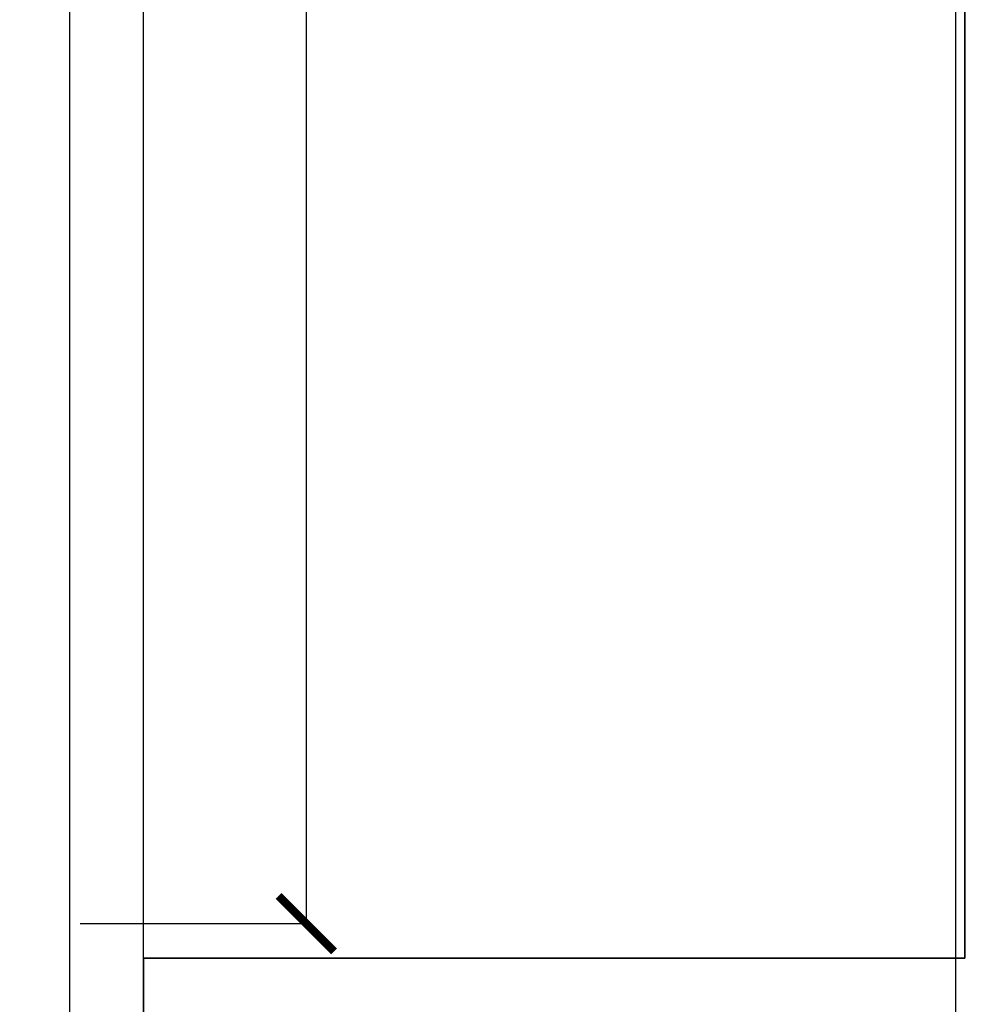
# Model space of a CAD drawing. Units: inches. Extents: x 844 to 2234, y 346 to 1084.
# Tile 6 of 93: x 1136 to 1189, y 627 to 680. Entities that reach past the tile are written whole.
import ezdxf

# ---------------------------------------------------------------- set-up
doc = ezdxf.new("R2010")
doc.units = ezdxf.units.IN
doc.header["$MEASUREMENT"] = 0
doc.layers.add('A-ANNO-DIMS', color=2, linetype='Continuous', lineweight=18)
doc.layers.add('A-WALL', color=7, linetype='Continuous', lineweight=35)
doc.styles.get("Standard").update_dxf_attribs({"font": 'arial.ttf'})
doc.dimstyles.get("Standard").update_dxf_attribs({"dimtxt": 6, "dimasz": 3, "dimexe": 0.18, "dimexo": 0.0625, "dimgap": 0.09, "dimtad": 0, "dimtih": 1, "dimtoh": 1, "dimdec": 1, "dimzin": 0, "dimdsep": 46, "dimlunit": 3, "dimtxsty": 'Standard', "dimblk": 'ARCHTICK', "dimcen": 0.09, "dimadec": 0, "dimazin": 0, "dimtfac": 1, "dimtdec": 1, "dimtofl": 0, "dimtmove": 0, "dimatfit": 3, "dimfxl": 1, "dimtolj": 1, "dimtzin": 0, "dimarcsym": 0})

# ---------------------------------------------------------------- blocks, each defined once
blk = doc.blocks.new('_ArchTick')
at = {"color": 0, "linetype": 'ByBlock', "const_width": 0.15}
blk.add_lwpolyline([(-0.5, -0.5), (0.5, 0.5)], dxfattribs=at)
blk = doc.blocks.new('*D54')
at = {"layer": 'A-ANNO-DIMS', "color": 0, "lineweight": -2, "transparency": 16777216}
for p, q in [((1139.678, 879.311), (1152.117, 879.311)), ((1151.937, 879.311), (1151.937, 758.401)), ((1151.937, 631.184), (1151.937, 752.094)), ((1139.678, 631.184), (1152.117, 631.184))]:
    blk.add_line(p, q, dxfattribs=at)
at = {"layer": 'Defpoints', "color": 0, "transparency": 16777216}
for p in [(1139.616, 879.311), (1139.616, 631.184), (1151.937, 631.184)]:
    blk.add_point(p, dxfattribs=at)
at = {"layer": 'A-ANNO-DIMS', "color": 0, "lineweight": -2, "transparency": 16777216, "xscale": 3, "yscale": 3, "zscale": 3}
for p, rotation in [((1151.937, 879.311), 90), ((1151.937, 631.184), 270)]:
    blk.add_blockref('_ArchTick', p, dxfattribs=dict(at, rotation=rotation))
at = {"layer": 'A-ANNO-DIMS', "color": 0, "transparency": 16777216, "insert": (1151.937, 755.248), "char_height": 6, "attachment_point": 5}
blk.add_mtext('\\A1;20\'-8.1"', dxfattribs=at)
blk = doc.blocks.new('*D143')
at = {"layer": 'A-ANNO-DIMS', "color": 0, "lineweight": -2, "transparency": 16777216}
for p, q in [((1139.116, 430.373), (1139.116, 1074.743)), ((1187.116, 430.373), (1187.116, 1074.743)), ((1139.116, 1074.563), (1154.93, 1074.563)), ((1187.116, 1074.563), (1171.301, 1074.563))]:
    blk.add_line(p, q, dxfattribs=at)
at = {"layer": 'Defpoints', "color": 0, "transparency": 16777216}
for p in [(1187.116, 1074.563), (1139.116, 430.311), (1187.116, 430.311)]:
    blk.add_point(p, dxfattribs=at)
at = {"layer": 'A-ANNO-DIMS', "color": 0, "lineweight": -2, "transparency": 16777216, "xscale": 3, "yscale": 3, "zscale": 3, "rotation": 180}
blk.add_blockref('_ArchTick', (1139.116, 1074.563), dxfattribs=at)
at = {"layer": 'A-ANNO-DIMS', "color": 0, "lineweight": -2, "transparency": 16777216, "xscale": 3, "yscale": 3, "zscale": 3}
blk.add_blockref('_ArchTick', (1187.116, 1074.563), dxfattribs=at)
at = {"layer": 'A-ANNO-DIMS', "color": 0, "transparency": 16777216, "insert": (1163.116, 1074.563), "char_height": 6, "attachment_point": 5}
blk.add_mtext('\\A1;4\'-0"', dxfattribs=at)
blk = doc.blocks.new('*D144')
at = {"layer": 'A-ANNO-DIMS', "color": 0, "lineweight": -2, "transparency": 16777216}
for p, q in [((1096.616, 439.373), (1096.616, 1074.743)), ((1143.116, 492.373), (1143.116, 1074.743)), ((1096.616, 1074.563), (1102.482, 1074.563)), ((1143.116, 1074.563), (1137.25, 1074.563))]:
    blk.add_line(p, q, dxfattribs=at)
at = {"layer": 'Defpoints', "color": 0, "transparency": 16777216}
for p in [(1143.116, 1074.563), (1143.116, 492.311), (1096.616, 439.311)]:
    blk.add_point(p, dxfattribs=at)
at = {"layer": 'A-ANNO-DIMS', "color": 0, "lineweight": -2, "transparency": 16777216, "xscale": 3, "yscale": 3, "zscale": 3, "rotation": 180}
blk.add_blockref('_ArchTick', (1096.616, 1074.563), dxfattribs=at)
at = {"layer": 'A-ANNO-DIMS', "color": 0, "lineweight": -2, "transparency": 16777216, "xscale": 3, "yscale": 3, "zscale": 3}
blk.add_blockref('_ArchTick', (1143.116, 1074.563), dxfattribs=at)
at = {"layer": 'A-ANNO-DIMS', "color": 0, "transparency": 16777216, "insert": (1119.866, 1074.563), "char_height": 6, "attachment_point": 5}
blk.add_mtext('\\A1;3\'-10 1/2"', dxfattribs=at)

msp = doc.modelspace()

# ---------------------------------------------------------------- linework, layer by layer
at = {"layer": 'A-WALL'}
for p, q in [((1187.616, 766.311), (1187.616, 629.311)), ((1143.116, 629.311), (1187.616, 629.311)), ((1143.116, 629.311), (1143.116, 516.311))]:
    msp.add_line(p, q, dxfattribs=at)

# ---------------------------------------------------------------- dimensions: what is measured, and where the dimension line sits
at = {"layer": 'A-ANNO-DIMS'}
for base, p1, p2, picture, middle in [((1143.116, 1074.563), (1096.616, 439.311), (1143.116, 492.311), '*D144', (1119.866, 1074.563)), ((1187.116, 1074.563), (1139.116, 430.311), (1187.116, 430.311), '*D143', (1163.116, 1074.563))]:
    dim = msp.add_linear_dim(base=base, p1=p1, p2=p2, dimstyle='Standard', override={"dimdec": 1, "dimlfac": 1, "dimrnd": 0, "dimzin": 1, "dimdsep": 46, "dimlunit": 4, "dimfrac": 2}, dxfattribs=at)
    dim.commit()
    dim.dimension.update_dxf_attribs({"geometry": picture, "text_midpoint": middle})
dim = msp.add_linear_dim(base=(1151.937, 631.184), p1=(1139.616, 879.311), p2=(1139.616, 631.184), angle=90, dimstyle='Standard', override={"dimclrd": 0, "dimclre": 0, "dimclrt": 0}, dxfattribs=at)
dim.commit()
dim.dimension.update_dxf_attribs({"geometry": '*D54', "text_midpoint": (1151.937, 755.248)})

doc.saveas('drawing.dxf')
